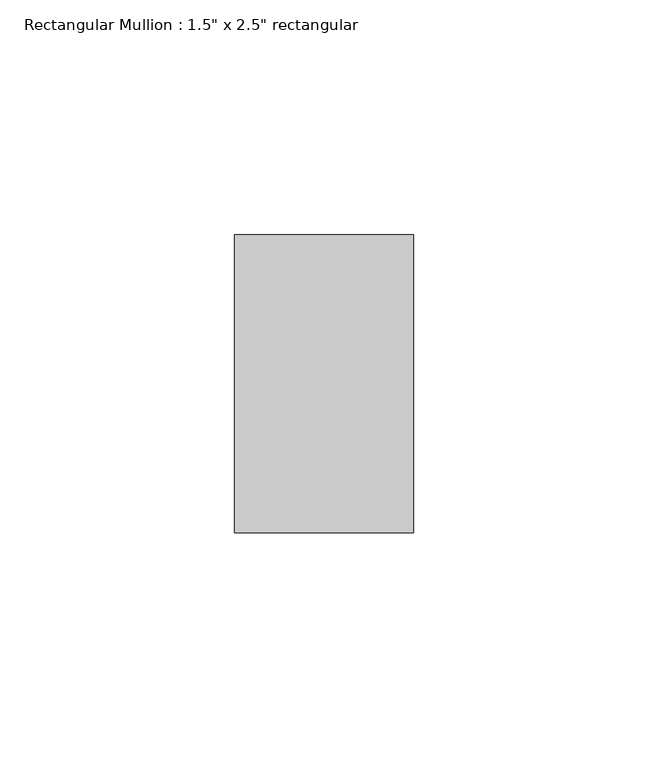
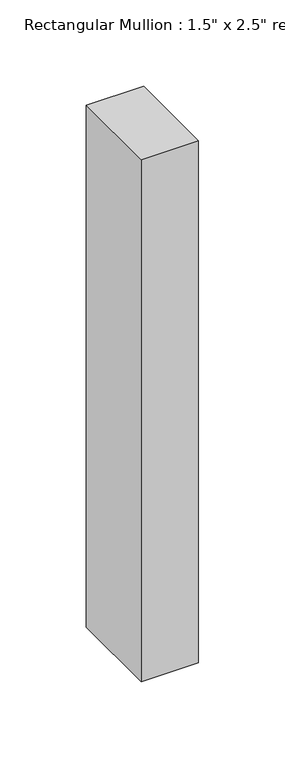
"""IFC4 building model written with IfcOpenShell, lengths in millimetres: member geometry."""

from ifc_helpers import new_model, si_unit, frame, origin, place, context, project, spatial, polyline, outline, extrude, source, transform, mapped, element, save


def member_bebcb7d7(model_context):
    return source(origin(), model_context, "Body", "SweptSolid", [
        extrude(outline(polyline([(0.0, 31.75), (0.0, -31.75), (-38.1, -31.75), (-38.1, 31.75), (0.0, 31.75)])), frame((0.0, 0.0, -368.3), z_axis=(0.0, 0.0, 1.0), x_axis=(1.0, 0.0, 0.0)), (0.0, 0.0, 1.0), 368.3),
    ])


if __name__ == "__main__":
    model = new_model("IFC4")
    model_context = context("Model", 3, world=origin())
    ifc_project = project(units=[si_unit("LENGTHUNIT", "METRE", prefix="MILLI")], contexts=[model_context])
    site = spatial("IfcSite", under=ifc_project)
    building = spatial("IfcBuilding", under=site)
    placement = place(None, origin())
    member_shape = member_bebcb7d7(model_context)
    element("IfcMember", 1, ObjectType="Rectangular Mullion : 1.5\" x 2.5\" rectangular", at=placement, inside=building, context=model_context, shape_type="MappedRepresentation", body=[
        mapped(member_shape, transform((0.0, 0.0, 0.0), x_axis=(1.0, 0.0, 0.0), y_axis=(0.0, 1.0, 0.0), z_axis=(0.0, 0.0, 1.0))),
    ])
    save(model, "model.ifc")

# Revit data of these elements
# Type "Rectangular Mullion : 1.5\" x 2.5\" rectangular"
#   built-in parameter 1007304 = 0.208333 (stored number, unit not read)
#   built-in parameter 1007301 = 0.0625 (stored number, unit not read)
#   built-in parameter 1007300 = 0.0625 (stored number, unit not read)
# Element 1 (IfcMember, "Rectangular Mullion : 1.5\" x 2.5\" rectangular")
#   Materials on its faces: "Damp-proofing"
# Materials
#   "Damp-proofing": class "Generic", colour RGB 127 127 127, transparency 0, Description = "Damp-proofing", Cost = 0
